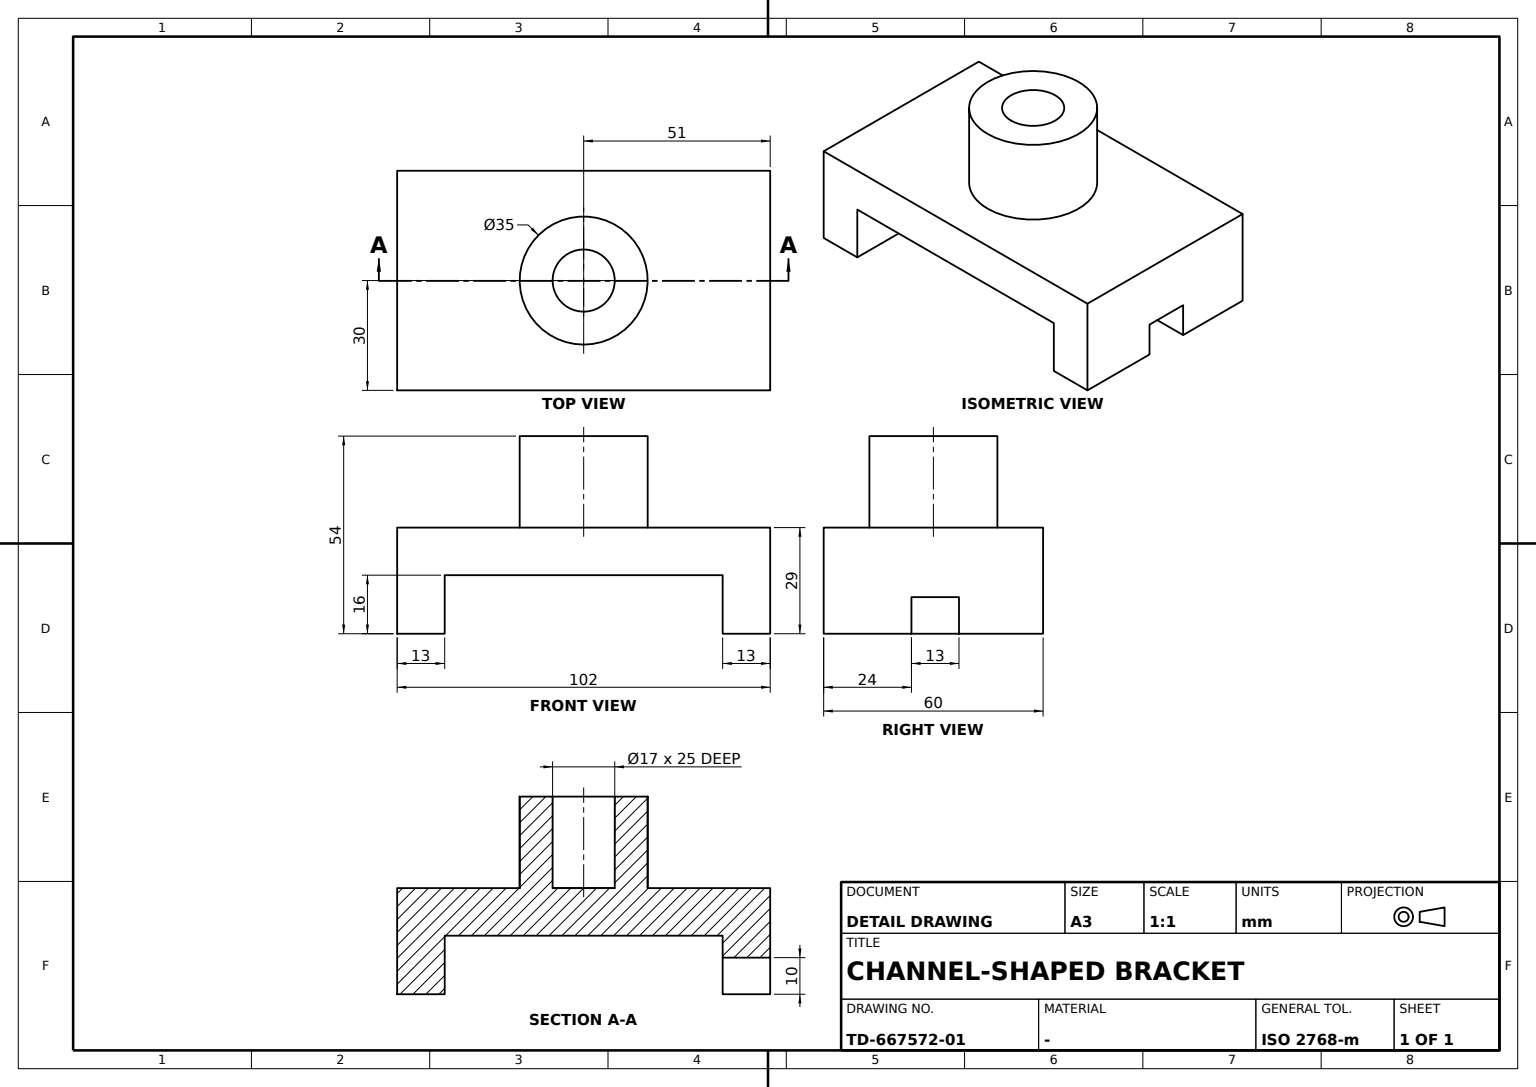
CATIA V5 part; units mm, degrees
sketch "Sketch1" plane through (0, 0, 0) normal (1, 0, 0) x (0, 1, 0)
  point P0 (-51, 0)
  line L0 (-51, 0) -> (51, 0)
  line L1 (51, 0) -> (51, -29)
  point P1 (51, -29)
  line L2 (51, -29) -> (38, -29)
  point P2 (38, -29)
  line L3 (38, -29) -> (38, -13)
  line L4 (38, -13) -> (-38, -13)
  line L5 (-38, -13) -> (-38, -29)
  point P3 (-38, -29)
  line L6 (-38, -29) -> (-51, -29)
  point P4 (-51, -29)
  line L7 (-51, -29) -> (-51, 0)
  dimension "distance L0 L4" = 13
  dimension "distance P2 P1" = 13
  dimension "distance P4 P3" = 13
  dimension "distance P4 P1" = 102
  dimension "distance P0 P4" = 29
  constraint coincidence P0 x-axis
  constraint coincidence P3 L2
  constraint horizontal L0 x-axis
  constraint horizontal L2 x-axis
  constraint horizontal L4 x-axis
  constraint horizontal L6 x-axis
  constraint vertical L1 y-axis
  constraint vertical L3 y-axis
  constraint vertical L5 y-axis
  constraint vertical L7 y-axis
  constraint symmetry L7 L1 y-axis
extrude "Pad1" add sketch "Sketch1" against normal blind 60
sketch "Sketch2" plane through (0, 51, 0) normal (0, 1, 0) x (-1, 0, 0)
  point P0 (24, -29)
  line L0 (24, -29) -> (24, -19)
  line L1 (24, -19) -> (37, -19)
  line L2 (37, -19) -> (37, -29)
  point P1 (37, -29)
  line L3 (0, -29) -> (60, -29) construction
  line L4 (0, -29) -> (60, -29) construction
  line L5 (24, -29) -> (37, -29)
  line L6 (0, -29) -> (0, 0) construction
  line L7 (0, -29) -> (0, 0) construction
  line L8 (60, -29) -> (60, 0) construction
  dimension "distance L6 L0" = 24
  dimension "distance L0 L2" = 13
  dimension "distance L7 L8" = 60
  constraint vertical L0 y-axis
  constraint vertical L2 y-axis
  constraint horizontal L1 x-axis
  constraint coincidence L3 P0
  constraint coincidence P1 L4
extrude "Pocket1" cut sketch "Sketch2" against normal blind 13
sketch "Sketch3" plane through (0, 0, 0) normal (0, 0, 1) x (1, 0, 0)
  circle A0 centre (-30, 0) radius 17.5
  point P0 (-30, 0)
  circle A1 centre (-30, 0) radius 8.5
  dimension "radius A1" = 8.5
  dimension "radius A0" = 17.5
  dimension "distance P0 y axis" = 30
  constraint coincidence P0 x-axis
extrude "Pad2" add sketch "Sketch3" along normal blind 25
